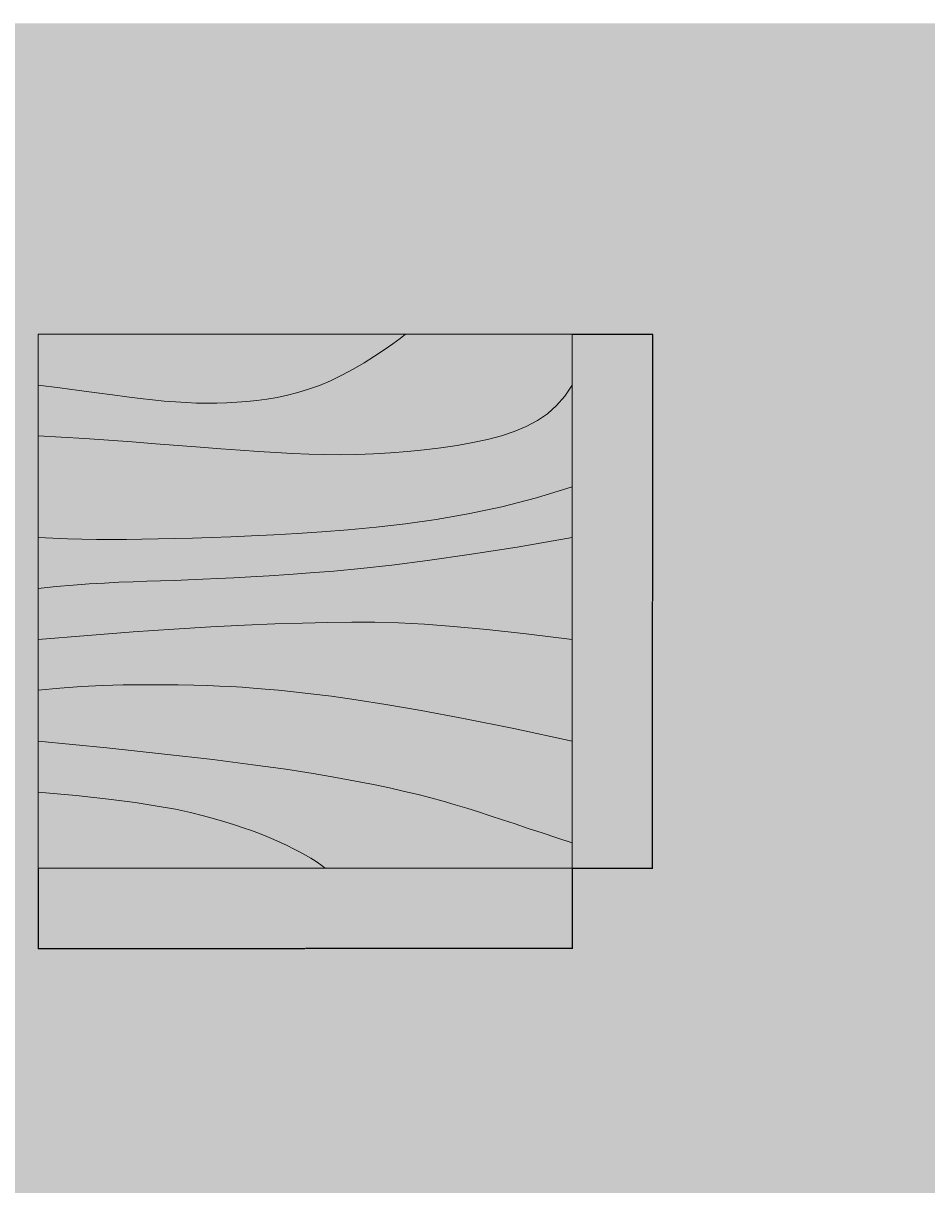
# Model space of a CAD drawing. Units: millimetres. Extents: x -229 to 16545, y -10488 to 4272.
# Tile 24 of 29: x 13075 to 13776, y -2111 to -1208. Entities that reach past the tile are written whole.
import ezdxf

# ---------------------------------------------------------------- set-up
doc = ezdxf.new("R2010")
doc.units = ezdxf.units.MM
for name, color, linetype, lineweight in [('A-ANNO-DIMS', 2, 'Continuous', 18), ('A-FURN', 8, 'Continuous', 18), ('A-FURN-PATT', 252, 'Continuous', 13)]:
    doc.layers.add(name, color=color, linetype=linetype, lineweight=lineweight)
doc.layers.add('A-FLOR-PATT', color=254, linetype='Continuous', lineweight=13, true_color=0xfeeab9)
doc.styles.get("Standard").update_dxf_attribs({"font": 'arial.ttf'})
doc.dimstyles.get("Standard").update_dxf_attribs({"dimtxt": 0.18, "dimasz": 0.18, "dimexe": 0.18, "dimexo": 0.0625, "dimgap": 0.09, "dimtad": 0, "dimtih": 1, "dimtoh": 1, "dimdec": 4, "dimzin": 0, "dimdsep": 46, "dimtxsty": 'Standard', "dimcen": 0.09, "dimadec": 0, "dimazin": 0, "dimtfac": 1, "dimtdec": 4, "dimtofl": 0, "dimtmove": 0, "dimatfit": 3, "dimfxl": 1, "dimtolj": 1, "dimtzin": 0, "dimarcsym": 0})

# ---------------------------------------------------------------- blocks, each defined once
blk = doc.blocks.new('Table - Square Woodgrain 42 x 42 in.')
blk.add_line((0, -42), (42, -42))
for points in [[(0, -4), (1.704, -4.2172), (3.2358, -4.4188), (4.615, -4.604), (5.8615, -4.7721), (6.9951, -4.9224), (8.0357, -5.0541), (9.0031, -5.1667), (9.9171, -5.2594), (10.7951, -5.3316), (11.6445, -5.3836), (12.4702, -5.4157), (13.277, -5.4283), (14.0698, -5.4217), (14.8535, -5.3964), (15.6331, -5.3526), (16.4133, -5.2908), (17.1986, -5.2103), (17.9913, -5.1062), (18.793, -4.9727), (19.6056, -4.8038), (20.4307, -4.5937), (21.2701, -4.3365), (22.1256, -4.0262), (22.9989, -3.6571), (23.888, -3.2272), (24.7756, -2.7516), (25.6408, -2.2491), (26.4624, -1.7387), (27.2195, -1.2395), (27.891, -0.7703), (28.456, -0.3501), (28.8934, 0.002)], [(0, -42), (0, 0), (42, 0), (42, -42)], [(0, -8), (1.8203, -8.1001), (3.6741, -8.2149), (5.5411, -8.3408), (7.4011, -8.4741), (9.2339, -8.6112), (11.0193, -8.7484), (12.7371, -8.8821), (14.3671, -9.0086), (15.8954, -9.1246), (17.3337, -9.2278), (18.6997, -9.3159), (20.0116, -9.387), (21.2871, -9.4389), (22.5442, -9.4696), (23.8008, -9.477), (25.0749, -9.459), (26.3791, -9.4137), (27.7049, -9.3403), (29.0383, -9.2382), (30.3655, -9.1068), (31.6728, -8.9455), (32.9461, -8.7535), (34.1717, -8.5304), (35.3358, -8.2756), (36.4268, -7.9863), (37.443, -7.6521), (38.3849, -7.2603), (39.253, -6.7986), (40.048, -6.2542), (40.7705, -5.6147), (41.421, -4.8674), (42, -4)], [(42, -12), (39.1784, -12.8621), (36.4519, -13.5654), (33.8246, -14.1294), (31.3004, -14.5731), (28.8832, -14.9161), (26.577, -15.1775), (24.3858, -15.3768), (22.3136, -15.5332), (20.3622, -15.6632), (18.5254, -15.7718), (16.7947, -15.8612), (15.1618, -15.9338), (13.6183, -15.9916), (12.1558, -16.0369), (10.7659, -16.0718), (9.4403, -16.0987), (8.1703, -16.1191), (6.9461, -16.1325), (5.7577, -16.1377), (4.595, -16.1335), (3.4479, -16.1188), (2.3064, -16.0924), (1.1604, -16.0532), (0, -16)], [(42, -16), (37.6529, -16.7365), (33.8802, -17.329), (30.6179, -17.7961), (27.8015, -18.1561), (25.3668, -18.4275), (23.2497, -18.6288), (21.3859, -18.7785), (19.7111, -18.8949), (18.1693, -18.9939), (16.7375, -19.0795), (15.401, -19.1534), (14.1449, -19.217), (12.9544, -19.2717), (11.8148, -19.3191), (10.7113, -19.3606), (9.6291, -19.3976), (8.5534, -19.4323), (7.47, -19.4689), (6.3643, -19.5122), (5.222, -19.5672), (4.0288, -19.6386), (2.7703, -19.7313), (1.4321, -19.8501), (0, -20)], [(0, -24), (3.9243, -23.6805), (7.4766, -23.4138), (10.6891, -23.1954), (13.5943, -23.0205), (16.2247, -22.8847), (18.6125, -22.7832), (20.7903, -22.7116), (22.7903, -22.6651), (24.6563, -22.642), (26.4764, -22.6507), (28.35, -22.7024), (30.3766, -22.8084), (32.6555, -22.98), (35.2861, -23.2283), (38.3678, -23.5645), (42, -24)], [(42, -32), (37.392, -31.017), (33.4585, -30.2231), (30.1291, -29.5949), (27.3334, -29.109), (25.0009, -28.742), (23.0612, -28.4707), (21.4439, -28.2716), (20.0786, -28.1215), (18.8998, -28.0002), (17.8609, -27.9014), (16.9206, -27.8219), (16.0371, -27.7588), (15.1691, -27.709), (14.2748, -27.6693), (13.3128, -27.6368), (12.2415, -27.6083), (11.0295, -27.5824), (9.6867, -27.5643), (8.233, -27.5608), (6.6884, -27.5787), (5.0728, -27.6248), (3.4062, -27.7058), (1.7086, -27.8286), (0, -28)], [(0, -32), (5.4026, -32.5358), (9.9494, -33.019), (13.7424, -33.4553), (16.8834, -33.8505), (19.4743, -34.2106), (21.6171, -34.5413), (23.4136, -34.8486), (24.9657, -35.1382), (26.3614, -35.4156), (27.6332, -35.6841), (28.7995, -35.9467), (29.8788, -36.2064), (30.8897, -36.4661), (31.8507, -36.7288), (32.7802, -36.9973), (33.6968, -37.2747), (34.6175, -37.5635), (35.5531, -37.8651), (36.5128, -38.1805), (37.506, -38.5108), (38.5421, -38.8568), (39.6302, -39.2197), (40.7797, -39.6004), (42, -40)], [(0, -36), (3.0098, -36.2857), (5.5354, -36.5643), (7.6368, -36.8359), (9.374, -37.1009), (10.807, -37.3597), (11.9957, -37.6126), (13.0002, -37.8599), (13.8804, -38.102), (14.6874, -38.3393), (15.4365, -38.5729), (16.1338, -38.8041), (16.7858, -39.0341), (17.3987, -39.264), (17.9787, -39.4952), (18.5322, -39.7288), (19.0655, -39.9662), (19.5832, -40.2081), (20.0842, -40.4544), (20.5657, -40.7046), (21.0249, -40.9581), (21.459, -41.2144), (21.8653, -41.4731), (22.2409, -41.7335), (22.5831, -41.9951)]]:
    blk.add_lwpolyline(points)
blk = doc.blocks.new('*D43')
at = {"layer": 'A-ANNO-DIMS', "color": 0, "lineweight": -2, "transparency": 16777216}
for p, q in [((13501.11, -1449.82), (13563.48, -1449.82)), ((13563.3, -1450), (13563.3, -1657.14)), ((13563.3, -1864.65), (13563.3, -1657.51)), ((13501.11, -1864.83), (13563.48, -1864.83))]:
    blk.add_line(p, q, dxfattribs=at)
at = {"layer": 'A-ANNO-DIMS', "color": 0, "transparency": 16777216}
for points in [[(13563.27, -1450), (13563.33, -1450), (13563.3, -1449.82)], [(13563.27, -1864.65), (13563.33, -1864.65), (13563.3, -1864.83)]]:
    blk.add_solid(points, dxfattribs=at)
at = {"layer": 'Defpoints', "color": 0, "transparency": 16777216}
for p in [(13501.05, -1449.82), (13563.3, -1449.82), (13501.05, -1864.83)]:
    blk.add_point(p, dxfattribs=at)
at = {"layer": 'A-ANNO-DIMS', "color": 0, "transparency": 16777216, "insert": (13563.3, -1657.33), "char_height": 0.18, "attachment_point": 5}
blk.add_mtext('\\A1;END TABLE 415', dxfattribs=at)
blk = doc.blocks.new('*D44')
at = {"layer": 'A-ANNO-DIMS', "color": 0, "lineweight": -2, "transparency": 16777216}
for p, q in [((13086.06, -1864.89), (13086.06, -1927.26)), ((13501.05, -1864.89), (13501.05, -1927.26)), ((13086.24, -1927.08), (13293.26, -1927.08)), ((13500.87, -1927.08), (13293.85, -1927.08))]:
    blk.add_line(p, q, dxfattribs=at)
at = {"layer": 'A-ANNO-DIMS', "color": 0, "transparency": 16777216}
for points in [[(13086.24, -1927.05), (13086.24, -1927.11), (13086.06, -1927.08)], [(13500.87, -1927.05), (13500.87, -1927.11), (13501.05, -1927.08)]]:
    blk.add_solid(points, dxfattribs=at)
at = {"layer": 'Defpoints', "color": 0, "transparency": 16777216}
for p in [(13086.06, -1864.83), (13501.05, -1864.83), (13501.05, -1927.08)]:
    blk.add_point(p, dxfattribs=at)
at = {"layer": 'A-ANNO-DIMS', "color": 0, "transparency": 16777216, "insert": (13293.55, -1927.08), "char_height": 0.18, "attachment_point": 5}
blk.add_mtext('\\A1;415', dxfattribs=at)

msp = doc.modelspace()

# ---------------------------------------------------------------- hatches: boundary and pattern name
at = {"layer": 'A-FLOR-PATT', "transparency": 33554592}
h = msp.add_hatch(color=256, dxfattribs=at)
h.dxf.hatch_style = 1
h.paths.add_polyline_path([(7975.933, -5325.772), (7943.121, -5325.772), (7943.121, -4576.49, 0.4014527), (7225.933, -5325.772, 0.4014527), (6508.746, -4576.49), (6508.746, -5325.772), (6475.933, -5325.772), (6475.933, -5438.272), (5975.933, -5438.272), (5975.933, -7267.724), (5975.933, -7438.272), (6478.619, -7438.272), (6463.448, -7355.919), (6464.88, -7356.837), (6463.849, -7358.097), (6478.619, -7438.272), (6610.327, -7438.272), (6632.656, -7409.564), (6632.525, -7406.967), (6634.208, -7407.569), (6619.273, -7426.77), (6654.466, -7438.272), (7610.517, -7438.272), (7607.41, -7421.409), (7608.842, -7422.327), (7607.812, -7423.587), (7610.517, -7438.272), (7975.933, -7438.272)])
h.paths.add_polyline_path([(13785.933, -1208.272), (9555.933, -1208.272), (9555.933, -961.785), (9705.933, -961.785), (9705.933, -918.035), (10704.976, -918.035, 0.4014527), (9705.933, 38.215), (9555.933, 38.215), (9555.933, 2021.728), (5975.933, 2021.728), (5975.933, 755.492), (5745.933, 755.492), (5745.933, 1427.266), (2918.813, 1427.266), (2918.813, -492.942), (5013.319, -492.942), (5013.319, -978.272), (5745.933, -978.272), (5745.933, -397.513), (5975.933, -397.513), (5975.933, -1208.272), (4560.933, -1208.272), (4560.933, -1265.772), (4448.433, -1265.772), (4448.433, -1298.585), (4445.933, -1298.585), (3699.151, -1298.585, 0.4014527), (4448.433, -2015.772), (4560.933, -2015.772), (4560.933, -2384.177), (5745.933, -2384.177), (5799.402, -2384.177), (5799.402, -4518.272), (5975.933, -4518.272), (5975.933, -5208.272), (6475.933, -5208.272), (6475.933, -4575.772), (6508.746, -4575.772), (6508.746, -4576.49, -0.3564726), (7216.672, -5208.272), (7235.194, -5208.272, -0.3564726), (7943.121, -4576.49), (7943.121, -4575.772), (7975.933, -4575.772), (7975.933, -5208.272), (11176.247, -5208.272), (11159.44, -5191.465), (10520.768, -5191.465), (10520.768, -4888.936), (10571.19, -4888.936), (10571.19, -4872.129), (10772.876, -4872.129), (10772.876, -4888.936), (10789.683, -4888.936), (10789.683, -4872.129), (10991.368, -4872.129), (10991.368, -4888.936), (11041.79, -4888.936), (11041.79, -4872.129), (11058.597, -4872.129, -0.0909091), (11428.354, -4872.129), (11445.162, -4872.129), (11445.162, -4888.936), (11529.197, -4888.936), (11529.197, -5191.465), (11327.512, -5191.465), (11310.704, -5208.272), (13785.933, -5208.272)])
h.paths.add_polyline_path([(11047.216, -1630.944, -1), (11402.816, -1630.944, -1)], flags=16)
h.paths.add_polyline_path([(11148.816, -1630.944), (11225.016, -1554.744), (11301.216, -1630.944), (11225.016, -1707.144)], flags=0)
h.paths.add_polyline_path([(11199.616, -1630.944, -1), (11250.416, -1630.944, -1)], flags=0)
h.paths.add_polyline_path([(11588.751, -2096.259), (11588.751, -1543.254, -0.266667), (12864.918, -1543.254), (12864.918, -2096.259), (12737.302, -2096.259), (12737.302, -2063.121), (11716.368, -2063.121), (11716.368, -2096.259)], flags=16)
h.paths.add_polyline_path([(12012.696, -2489.42), (12600.997, -2489.42), (12600.997, -3666.022), (12012.696, -3666.022)], flags=16)
h.paths.add_polyline_path([(12176.41, -3599.403), (12174.938, -3609.076), (12173.789, -3618.819), (12173.09, -3628.559), (12172.973, -3638.221), (12173.89, -3652.852), (12175.008, -3657.025), (12172.909, -3643.473), (12173.142, -3624.297), (12175.386, -3605.273)], flags=0)
h.paths.add_polyline_path([(8026.289, -286.944), (7737.703, -287.19), (7734.87, -269.156), (8029.092, -268.905)], flags=16)
h.paths.add_polyline_path([(7733.453, -260.139), (7710.784, -115.865), (7557.191, -115.996), (7556.999, 109.744), (7412.687, 132.166), (7412.433, 429.206), (7556.707, 451.876), (7556.568, 614.769), (7412.256, 637.19), (7412.003, 934.231), (7556.276, 956.9), (7556.084, 1182.639), (7709.677, 1182.77), (7732.099, 1327.082), (8029.14, 1327.335), (8051.808, 1183.062), (8205.401, 1183.192), (8205.594, 957.454), (8349.906, 935.031), (8350.159, 637.99), (8205.885, 615.322), (8206.024, 452.43), (8350.336, 430.006), (8350.59, 132.965), (8206.316, 110.298), (8206.509, -115.442), (8052.916, -115.573), (8030.493, -259.885)], flags=16)
h.paths.add_polyline_path([(12261.416, -3475.554), (12262.632, -3486.776), (12264.032, -3497.007), (12265.554, -3506.365), (12267.136, -3514.968), (12268.719, -3522.935), (12271.304, -3535.59), (12273.606, -3548.078), (12275.271, -3561.064), (12275.93, -3574.938), (12275.325, -3590.3), (12273.425, -3607.964), (12270.795, -3625.658), (12268.066, -3641.063), (12266.318, -3649.679), (12265.456, -3653.626), (12263.984, -3659.846), (12264.032, -3659.566), (12264.342, -3658.241), (12264.807, -3656.37), (12265.456, -3653.626), (12266.318, -3649.679), (12267.409, -3644.302), (12268.668, -3637.664), (12270.019, -3630.037), (12271.384, -3621.695), (12272.69, -3612.908), (12273.857, -3603.948), (12274.81, -3595.088), (12275.47, -3586.601), (12275.782, -3578.689), (12275.757, -3571.292), (12275.423, -3564.275), (12274.816, -3557.512), (12273.964, -3550.872), (12272.896, -3544.224), (12271.645, -3537.439), (12270.24, -3530.385), (12267.543, -3517.181), (12264.612, -3501.247), (12261.849, -3481.059)], flags=0)
h.paths.add_polyline_path([(12332.136, -3408.03), (12333.483, -3416.79), (12335.077, -3424.54), (12336.915, -3431.355), (12338.991, -3437.32), (12341.266, -3442.55), (12343.694, -3447.166), (12346.229, -3451.292), (12348.826, -3455.051), (12351.438, -3458.563), (12357.476, -3466.491), (12363.61, -3476.575), (12368.309, -3489.762), (12369.929, -3503.427), (12369.842, -3516.511), (12368.43, -3530.867), (12365.816, -3545.835), (12362.382, -3559.786), (12360.968, -3564.487), (12363.063, -3557.021), (12364.898, -3549.566), (12366.473, -3542.077), (12367.773, -3534.631), (12368.781, -3527.301), (12369.483, -3520.162), (12369.863, -3513.291), (12369.906, -3506.759), (12369.599, -3500.643), (12368.93, -3494.999), (12367.924, -3489.796), (12366.61, -3484.994), (12365.024, -3480.542), (12363.19, -3476.399), (12361.141, -3472.516), (12358.909, -3468.847), (12356.525, -3465.347), (12354.02, -3461.954), (12351.438, -3458.563), (12345.462, -3450.529), (12339.923, -3439.996), (12335.85, -3428.296), (12332.68, -3412.888)], flags=0)
h.paths.add_polyline_path([(12385.287, -3334.612), (12384.977, -3342.409), (12385.02, -3349.196), (12385.4, -3355.066), (12386.104, -3360.105), (12387.112, -3364.41), (12388.412, -3368.071), (12389.987, -3371.181), (12391.823, -3373.832), (12393.919, -3376.097), (12396.337, -3377.978), (12399.153, -3379.462), (12402.445, -3380.531), (12406.289, -3381.172), (12410.758, -3381.371), (12415.935, -3381.106), (12421.893, -3380.368), (12428.658, -3379.159), (12436.069, -3377.55), (12443.907, -3375.635), (12451.961, -3373.505), (12460.015, -3371.254), (12467.853, -3368.971), (12475.263, -3366.749), (12482.029, -3364.68), (12491.877, -3361.657), (12497.701, -3360.107), (12501.639, -3359.288), (12510.135, -3358.326), (12519.662, -3365.412), (12524.243, -3378.911), (12523.764, -3390.7), (12520.746, -3401.577), (12514.248, -3415.634), (12511.518, -3420.418), (12515.856, -3412.154), (12519.153, -3405.024), (12521.516, -3398.804), (12523.049, -3393.276), (12523.865, -3388.212), (12524.059, -3383.441), (12523.7, -3378.958), (12522.853, -3374.815), (12521.576, -3371.054), (12519.931, -3367.722), (12517.982, -3364.865), (12515.786, -3362.529), (12513.405, -3360.758), (12510.877, -3359.588), (12508.136, -3358.982), (12505.086, -3358.897), (12501.639, -3359.288), (12497.701, -3360.107), (12493.183, -3361.309), (12487.988, -3362.851), (12476.403, -3366.408), (12463.335, -3370.326), (12447.372, -3374.788), (12431.759, -3378.604), (12418.504, -3380.974), (12405.811, -3381.624), (12394.725, -3378.025), (12388.039, -3368.367), (12385.583, -3357.877), (12384.826, -3346.204), (12385.428, -3331.059), (12385.953, -3325.719)], flags=0)
h.paths.add_polyline_path([(7880.016, 1173.969), (7880.373, 1175.495), (7880.433, 1175.851), (7879.484, 1171.818)], flags=0)
h.paths.add_polyline_path([(7802.33, 874.962), (7800.771, 885.032), (7798.932, 893.941), (7796.811, 901.774), (7794.419, 908.63), (7791.798, 914.639), (7789.002, 919.945), (7786.083, 924.686), (7783.093, 929.005), (7780.087, 933.043), (7774.996, 939.717), (7768.406, 949.37), (7762.174, 963.427), (7759.342, 978.002), (7758.629, 991.888), (7759.492, 1007.928), (7761.801, 1025.496), (7765.392, 1044.035), (7766.625, 1049.048), (7764.522, 1039.543), (7762.719, 1030.232), (7761.232, 1021.168), (7760.08, 1012.405), (7759.28, 1003.994), (7758.849, 995.988), (7758.806, 988.44), (7759.167, 981.404), (7759.942, 974.914), (7761.104, 968.936), (7762.617, 963.414), (7764.448, 958.299), (7766.559, 953.535), (7768.918, 949.073), (7771.487, 944.856), (7774.232, 940.835), (7777.115, 936.938), (7782.377, 930.041), (7787.845, 922.139), (7793.348, 911.698), (7798.042, 898.247), (7801.702, 880.527)], flags=0)
h.paths.add_polyline_path([(12519.068, -3228.534), (12519.615, -3236.235), (12520.529, -3242.343), (12521.78, -3247.103), (12523.337, -3250.758), (12525.171, -3253.556), (12527.248, -3255.709), (12529.522, -3257.296), (12531.95, -3258.361), (12534.486, -3258.949), (12537.082, -3259.11), (12539.694, -3258.888), (12542.277, -3258.329), (12544.781, -3257.478), (12547.173, -3256.388), (12549.46, -3255.129), (12550.455, -3254.517), (12555.825, -3251.109), (12557.835, -3249.942), (12565.181, -3246.404), (12574.565, -3253.032), (12576.931, -3265.022), (12576.627, -3277.425), (12575.416, -3290.819), (12574.851, -3295.392), (12575.708, -3287.593), (12576.322, -3280.806), (12576.688, -3274.939), (12576.812, -3269.899), (12576.688, -3265.593), (12576.322, -3261.932), (12575.708, -3258.822), (12574.851, -3256.172), (12573.753, -3253.905), (12572.439, -3252.005), (12570.943, -3250.474), (12569.293, -3249.309), (12567.523, -3248.513), (12565.658, -3248.083), (12563.732, -3248.022), (12561.777, -3248.328), (12559.814, -3248.989), (12557.835, -3249.942), (12555.825, -3251.109), (12553.77, -3252.413), (12551.652, -3253.78), (12549.46, -3255.129), (12543.167, -3258.594), (12532.661, -3259.485), (12524.685, -3253.923), (12520.949, -3245.152), (12519.138, -3233.042)], flags=0)
h.paths.add_polyline_path([(7741.293, 790.501), (7741.641, 799.467), (7741.584, 807.269), (7741.141, 814.015), (7740.329, 819.809), (7739.165, 824.757), (7737.667, 828.966), (7735.853, 832.541), (7733.74, 835.586), (7731.348, 838.188), (7728.71, 840.348), (7725.861, 842.052), (7722.836, 843.28), (7719.671, 844.015), (7716.4, 844.237), (7713.06, 843.932), (7709.684, 843.081), (7706.304, 841.686), (7702.923, 839.834), (7699.543, 837.629), (7696.164, 835.178), (7692.784, 832.585), (7684.718, 826.315), (7675.609, 820.63), (7664.001, 817.274), (7654.105, 821.884), (7647.171, 832.02), (7644.191, 846.522), (7646.321, 860.288), (7647.49, 864.223), (7645.946, 857.865), (7645.046, 852.044), (7644.827, 846.557), (7645.243, 841.404), (7646.221, 836.642), (7647.693, 832.318), (7649.587, 828.489), (7651.832, 825.206), (7654.359, 822.523), (7657.097, 820.49), (7659.984, 819.145), (7662.993, 818.452), (7666.108, 818.357), (7669.311, 818.809), (7672.583, 819.755), (7675.908, 821.139), (7679.268, 822.913), (7682.645, 825.021), (7686.025, 827.401), (7689.404, 829.958), (7692.784, 832.585), (7700.505, 838.509), (7709.871, 843.64), (7721.436, 844.698), (7733.277, 837.617), (7739.571, 825.214), (7741.557, 811.049), (7741.669, 795.575)], flags=0)
h.paths.add_polyline_path([(8377.641, 137.216), (8359.607, 134.382), (8359.356, 428.605), (8377.395, 425.802)], flags=16)
h.paths.add_polyline_path([(7650.715, 668.465), (7650.08, 677.319), (7649.023, 684.34), (7647.579, 689.811), (7645.785, 694.012), (7643.675, 697.228), (7641.286, 699.7), (7638.669, 701.521), (7635.876, 702.744), (7632.96, 703.419), (7629.974, 703.601), (7626.971, 703.344), (7624.004, 702.697), (7621.125, 701.717), (7618.375, 700.462), (7615.749, 699.013), (7614.561, 698.279), (7608.435, 694.382), (7606.125, 693.04), (7598.981, 689.594), (7589.669, 693.773), (7585.26, 702.856), (7584.221, 713.11), (7584.49, 724.584), (7585.863, 739.937), (7586.518, 745.277), (7585.539, 736.31), (7584.841, 728.507), (7584.424, 721.761), (7584.288, 715.966), (7584.433, 711.016), (7584.86, 706.807), (7585.567, 703.231), (7586.556, 700.186), (7587.821, 697.58), (7589.332, 695.397), (7591.053, 693.637), (7592.951, 692.3), (7594.989, 691.385), (7597.132, 690.895), (7599.346, 690.826), (7601.594, 691.18), (7603.851, 691.943), (7606.125, 693.04), (7608.435, 694.382), (7610.797, 695.885), (7613.229, 697.458), (7620.475, 701.929), (7632.001, 704.44), (7643.476, 699.417), (7648.536, 687.571), (7650.63, 673.661)], flags=0)
h.paths.add_polyline_path([(7385.628, 136.37), (7385.382, 424.956), (7403.416, 427.789), (7403.667, 133.567)], flags=16)
h.paths.add_polyline_path([(12993.884, -2257.186), (12959.588, -2257.186), (12959.588, -2125.099), (13531.966, -2125.099, -0.1904762), (13531.966, -3974.321), (12959.588, -3974.321), (12959.588, -3842.233), (12993.884, -3842.233)], flags=16)
h.paths.add_polyline_path([(13413.486, -3313.884), (13413.486, -2785.535), (13562.885, -2785.535, -0.0496282), (13562.885, -3313.884)], flags=0)
h.paths.add_polyline_path([(8377.21, 642.241), (8359.176, 639.407), (8358.925, 933.629), (8376.964, 930.826)], flags=16)
h.paths.add_polyline_path([(13086.058, -1864.83), (13086.058, -1449.84), (13501.048, -1449.84), (13501.048, -1864.83)], flags=16)
h.paths.add_polyline_path([(13305.814, -1862.197), (13302.103, -1859.624), (13298.088, -1857.068), (13293.799, -1854.536), (13289.262, -1852.031), (13284.504, -1849.559), (13279.554, -1847.125), (13274.439, -1844.735), (13269.17, -1842.389), (13263.701, -1840.081), (13257.97, -1837.797), (13251.914, -1835.525), (13245.472, -1833.252), (13238.582, -1830.968), (13231.18, -1828.66), (13223.206, -1826.315), (13209.182, -1822.458), (13204.584, -1821.48), (13217.962, -1824.773), (13235.072, -1829.804), (13248.777, -1834.349), (13260.829, -1838.869), (13274.479, -1844.63), (13289.675, -1852.101), (13302.553, -1859.704)], flags=0)
h.paths.add_polyline_path([(13428.104, -1820.994), (13419.007, -1818.141), (13409.95, -1815.4), (13400.766, -1812.747), (13391.271, -1810.151), (13376.087, -1806.251), (13370.618, -1805.019), (13386.304, -1808.794), (13405.087, -1813.928), (13423.014, -1819.354)], flags=0)
h.paths.add_polyline_path([(7385.197, 641.395), (7384.951, 929.98), (7402.986, 932.814), (7403.236, 638.592)], flags=16)
h.paths.add_polyline_path([(13262.537, -1725.526), (13253.246, -1724.74), (13244.516, -1724.117), (13235.94, -1723.625), (13223.267, -1723.062), (13217.598, -1722.912), (13231.966, -1723.397), (13248.733, -1724.359), (13266.899, -1725.895), (13272.802, -1726.502)], flags=0)
h.paths.add_polyline_path([(13191.893, -1641.137), (13208.675, -1640.506), (13214.057, -1640.258), (13197.763, -1640.936)], flags=0)
h.paths.add_polyline_path([(13097.524, -1608.457), (13114.284, -1609.031), (13120.126, -1609.105), (13103.045, -1608.71)], flags=0)
h.paths.add_polyline_path([(13465.328, -1521.577), (13473.906, -1517.015), (13481.761, -1511.636), (13492.562, -1502.076), (13495.327, -1497.933), (13485.818, -1508.858), (13470.208, -1519.547)], flags=0)
h.paths.add_polyline_path([(13175.015, -1500.891), (13184.046, -1501.807), (13192.721, -1502.52), (13201.114, -1503.034), (13209.273, -1503.351), (13217.244, -1503.476), (13225.078, -1503.41), (13232.821, -1503.16), (13240.524, -1502.728), (13248.233, -1502.117), (13255.993, -1501.322), (13263.825, -1500.293), (13271.746, -1498.974), (13279.775, -1497.305), (13287.928, -1495.229), (13296.222, -1492.688), (13304.675, -1489.622), (13313.304, -1485.975), (13322.089, -1481.727), (13330.859, -1477.028), (13339.408, -1472.063), (13347.526, -1467.02), (13355.006, -1462.087), (13364.86, -1455.202), (13367.224, -1453.299), (13358.544, -1459.754), (13343.348, -1469.775), (13326.143, -1479.767), (13309.023, -1488.045), (13292.249, -1494.129), (13276.009, -1498.264), (13260.299, -1500.88), (13244.401, -1502.51), (13228.945, -1503.378), (13213.316, -1503.508), (13197.047, -1502.876), (13180.088, -1501.481)], flags=0)
h.paths.add_polyline_path([(7733.501, 1336.101), (7736.303, 1354.14), (8024.889, 1354.386), (8027.723, 1336.352)], flags=16)
at = {"layer": 'A-FURN-PATT', "transparency": 33554569}
h = msp.add_hatch(color=256, dxfattribs=at)
h.dxf.hatch_style = 1
h.paths.add_polyline_path([(12600.997, -2489.42), (12553.933, -2489.42), (12553.58, -2583.852), (12552.584, -2666.503), (12551.036, -2738.644), (12549.03, -2801.547), (12546.656, -2856.483), (12544.004, -2904.723), (12541.171, -2947.542), (12538.245, -2986.207), (12535.313, -3021.787), (12532.444, -3054.526), (12529.695, -3084.461), (12527.132, -3111.629), (12524.814, -3136.073), (12522.802, -3157.826), (12521.157, -3176.928), (12519.941, -3193.42), (12519.202, -3207.371), (12518.921, -3218.994), (12519.068, -3228.534), (12519.615, -3236.235), (12520.529, -3242.343), (12521.78, -3247.103), (12523.337, -3250.758), (12525.171, -3253.556), (12527.248, -3255.709), (12529.522, -3257.296), (12531.95, -3258.361), (12534.486, -3258.949), (12537.082, -3259.11), (12539.694, -3258.888), (12542.277, -3258.329), (12544.781, -3257.478), (12547.173, -3256.388), (12549.46, -3255.129), (12551.652, -3253.78), (12559.563, -3248.675), (12566.794, -3247.543), (12572.687, -3251.706), (12575.978, -3258.498), (12576.872, -3267.431), (12576.627, -3277.425), (12575.708, -3287.593), (12574.851, -3295.392), (12573.749, -3304.309), (12572.419, -3314.522), (12570.874, -3326.221), (12569.131, -3339.597), (12567.203, -3354.842), (12565.107, -3372.146), (12562.857, -3391.705), (12560.469, -3413.705), (12557.959, -3438.275), (12555.343, -3465.264), (12552.633, -3494.46), (12549.848, -3525.645), (12547.001, -3558.61), (12544.106, -3593.137), (12541.184, -3629.012), (12538.245, -3666.022), (12600.997, -3666.022)])
h.paths.add_polyline_path([(12544.004, -2904.723), (12546.656, -2856.483), (12549.03, -2801.547), (12551.036, -2738.644), (12552.584, -2666.503), (12553.58, -2583.852), (12553.933, -2489.42), (12420.585, -2489.42), (12422.824, -2618.374), (12423.791, -2723.534), (12423.687, -2808.136), (12422.708, -2875.41), (12421.057, -2928.591), (12418.93, -2970.907), (12416.527, -3005.595), (12414.049, -3035.885), (12411.656, -3064.467), (12409.37, -3091.846), (12407.177, -3117.984), (12405.059, -3142.842), (12403.004, -3166.384), (12400.994, -3188.569), (12399.016, -3209.359), (12397.053, -3228.718), (12395.1, -3246.62), (12393.191, -3263.097), (12391.376, -3278.194), (12389.699, -3291.961), (12388.205, -3304.438), (12386.942, -3315.677), (12385.953, -3325.719), (12385.287, -3334.612), (12384.977, -3342.409), (12385.02, -3349.196), (12385.4, -3355.066), (12386.104, -3360.105), (12387.112, -3364.41), (12388.412, -3368.071), (12389.987, -3371.181), (12391.823, -3373.832), (12393.919, -3376.097), (12396.337, -3377.978), (12399.153, -3379.462), (12402.445, -3380.531), (12406.289, -3381.172), (12410.758, -3381.371), (12415.935, -3381.106), (12421.893, -3380.368), (12428.658, -3379.159), (12436.069, -3377.55), (12443.907, -3375.635), (12451.961, -3373.505), (12460.015, -3371.254), (12467.853, -3368.971), (12475.263, -3366.749), (12482.029, -3364.68), (12491.877, -3361.657), (12502.516, -3358.826), (12511.128, -3359.064), (12517.01, -3363.44), (12520.955, -3369.223), (12523.527, -3376.802), (12524.25, -3385.824), (12522.632, -3395.865), (12519.153, -3405.024), (12515.856, -3412.154), (12511.518, -3420.418), (12506.031, -3430.037), (12499.288, -3441.236), (12491.181, -3454.234), (12481.682, -3469.286), (12471.081, -3486.774), (12459.744, -3507.112), (12448.039, -3530.713), (12436.334, -3557.99), (12424.997, -3589.358), (12414.396, -3625.231), (12404.897, -3666.022), (12538.245, -3666.022), (12541.184, -3629.012), (12544.106, -3593.137), (12547.001, -3558.61), (12549.848, -3525.645), (12552.633, -3494.46), (12555.343, -3465.264), (12557.959, -3438.275), (12560.469, -3413.705), (12562.857, -3391.705), (12565.107, -3372.146), (12567.203, -3354.842), (12569.131, -3339.597), (12570.874, -3326.221), (12572.419, -3314.522), (12573.749, -3304.309), (12574.851, -3295.392), (12575.708, -3287.593), (12576.322, -3280.806), (12576.688, -3274.939), (12576.812, -3269.899), (12576.688, -3265.593), (12576.322, -3261.932), (12575.708, -3258.822), (12574.851, -3256.172), (12573.753, -3253.905), (12572.439, -3252.005), (12570.943, -3250.474), (12569.293, -3249.309), (12567.523, -3248.513), (12565.658, -3248.083), (12563.732, -3248.022), (12561.777, -3248.328), (12559.814, -3248.989), (12557.835, -3249.942), (12555.825, -3251.109), (12553.77, -3252.413), (12547.19, -3256.659), (12539.533, -3259.262), (12531.64, -3258.773), (12524.685, -3253.923), (12520.949, -3245.152), (12519.615, -3236.235), (12519.068, -3228.534), (12518.921, -3218.994), (12519.202, -3207.371), (12519.941, -3193.42), (12521.157, -3176.928), (12522.802, -3157.826), (12524.814, -3136.073), (12527.132, -3111.629), (12529.695, -3084.461), (12532.444, -3054.526), (12535.313, -3021.787), (12538.245, -2986.207), (12541.171, -2947.542)])
h.paths.add_polyline_path([(12418.93, -2970.907), (12421.057, -2928.591), (12422.708, -2875.41), (12423.687, -2808.136), (12423.791, -2723.534), (12422.824, -2618.374), (12420.585, -2489.42), (12349.989, -2489.42), (12347.396, -2591.092), (12345.433, -2678.094), (12343.99, -2752.122), (12342.962, -2814.864), (12342.239, -2868.017), (12341.715, -2913.271), (12341.284, -2952.323), (12340.837, -2986.86), (12340.288, -3018.358), (12339.633, -3047.386), (12338.883, -3074.301), (12338.06, -3099.455), (12337.173, -3123.199), (12336.242, -3145.885), (12335.279, -3167.868), (12334.301, -3189.498), (12333.326, -3211.038), (12332.381, -3232.395), (12331.496, -3253.384), (12330.706, -3273.821), (12330.037, -3293.523), (12329.52, -3312.306), (12329.188, -3329.984), (12329.071, -3346.378), (12329.194, -3361.343), (12329.561, -3374.915), (12330.175, -3387.169), (12331.032, -3398.18), (12332.136, -3408.03), (12333.483, -3416.79), (12335.077, -3424.54), (12336.915, -3431.355), (12338.991, -3437.32), (12341.266, -3442.55), (12343.694, -3447.166), (12346.229, -3451.292), (12348.826, -3455.051), (12351.438, -3458.563), (12357.476, -3466.491), (12362.356, -3474.514), (12365.989, -3482.725), (12368.611, -3492.308), (12369.929, -3503.427), (12369.863, -3513.291), (12369.483, -3520.162), (12368.781, -3527.301), (12367.773, -3534.631), (12366.473, -3542.077), (12364.898, -3549.566), (12363.063, -3557.021), (12360.968, -3564.487), (12358.568, -3572.468), (12355.799, -3581.585), (12352.603, -3592.463), (12348.916, -3605.723), (12344.678, -3621.988), (12339.827, -3641.88), (12334.301, -3666.022), (12404.897, -3666.022), (12414.396, -3625.231), (12424.997, -3589.358), (12436.334, -3557.99), (12448.039, -3530.713), (12459.744, -3507.112), (12471.081, -3486.774), (12481.682, -3469.286), (12491.181, -3454.234), (12499.288, -3441.236), (12506.031, -3430.037), (12511.518, -3420.418), (12515.856, -3412.154), (12519.153, -3405.024), (12521.516, -3398.804), (12523.049, -3393.276), (12523.865, -3388.212), (12524.059, -3383.441), (12523.7, -3378.958), (12522.853, -3374.815), (12521.576, -3371.054), (12519.931, -3367.722), (12517.982, -3364.865), (12515.786, -3362.529), (12513.405, -3360.758), (12510.877, -3359.588), (12508.136, -3358.982), (12505.086, -3358.897), (12501.639, -3359.288), (12497.701, -3360.107), (12493.183, -3361.309), (12487.988, -3362.851), (12476.403, -3366.408), (12463.335, -3370.326), (12451.961, -3373.505), (12439.372, -3376.834), (12424.661, -3380.026), (12412.995, -3381.47), (12402.039, -3380.984), (12393.748, -3376.613), (12389.022, -3369.787), (12386.442, -3362.522), (12385.041, -3352.492), (12384.977, -3342.409), (12385.287, -3334.612), (12385.953, -3325.719), (12386.942, -3315.677), (12388.205, -3304.438), (12389.699, -3291.961), (12391.376, -3278.194), (12393.191, -3263.097), (12395.1, -3246.62), (12397.053, -3228.718), (12399.016, -3209.359), (12400.994, -3188.569), (12403.004, -3166.384), (12405.059, -3142.842), (12407.177, -3117.984), (12409.37, -3091.846), (12411.656, -3064.467), (12414.049, -3035.885), (12416.527, -3005.595)])
h.paths.add_polyline_path([(12340.837, -2986.86), (12341.284, -2952.323), (12341.715, -2913.271), (12342.239, -2868.017), (12342.962, -2814.864), (12343.99, -2752.122), (12345.433, -2678.094), (12347.396, -2591.092), (12349.989, -2489.42), (12248.016, -2489.42), (12253.364, -2589.902), (12257.71, -2678.871), (12261.149, -2757.499), (12263.787, -2826.958), (12265.718, -2888.42), (12267.044, -2943.055), (12267.866, -2992.039), (12268.279, -3036.54), (12268.378, -3077.58), (12268.209, -3115.572), (12267.809, -3150.776), (12267.219, -3183.452), (12266.473, -3213.86), (12265.614, -3242.261), (12264.679, -3268.917), (12263.704, -3294.084), (12262.732, -3317.981), (12261.804, -3340.639), (12260.969, -3362.039), (12260.273, -3382.167), (12259.759, -3401.008), (12259.477, -3418.547), (12259.469, -3434.769), (12259.782, -3449.659), (12260.445, -3463.221), (12261.416, -3475.554), (12262.632, -3486.776), (12264.032, -3497.007), (12265.554, -3506.365), (12267.136, -3514.968), (12268.719, -3522.935), (12271.304, -3535.59), (12273.606, -3548.078), (12275.271, -3561.064), (12275.757, -3571.292), (12275.782, -3578.689), (12275.47, -3586.601), (12274.81, -3595.088), (12273.857, -3603.948), (12272.69, -3612.908), (12271.384, -3621.695), (12270.019, -3630.037), (12268.066, -3641.063), (12265.651, -3652.97), (12264.342, -3658.241), (12264.032, -3659.566), (12263.842, -3660.678), (12263.746, -3661.906), (12263.708, -3663.576), (12263.704, -3666.022), (12334.301, -3666.022), (12339.827, -3641.88), (12344.678, -3621.988), (12348.916, -3605.723), (12352.603, -3592.463), (12355.799, -3581.585), (12358.568, -3572.468), (12360.968, -3564.487), (12363.063, -3557.021), (12364.898, -3549.566), (12366.473, -3542.077), (12367.773, -3534.631), (12368.781, -3527.301), (12369.483, -3520.162), (12369.863, -3513.291), (12369.906, -3506.759), (12369.599, -3500.643), (12368.93, -3494.999), (12367.924, -3489.796), (12366.61, -3484.994), (12365.024, -3480.542), (12363.19, -3476.399), (12361.141, -3472.516), (12358.909, -3468.847), (12356.525, -3465.347), (12354.02, -3461.954), (12347.609, -3453.536), (12342.257, -3444.828), (12337.759, -3434.488), (12335.077, -3424.54), (12333.483, -3416.79), (12332.136, -3408.03), (12331.032, -3398.18), (12330.175, -3387.169), (12329.561, -3374.915), (12329.194, -3361.343), (12329.071, -3346.378), (12329.188, -3329.984), (12329.52, -3312.306), (12330.037, -3293.523), (12330.706, -3273.821), (12331.496, -3253.384), (12332.381, -3232.395), (12333.326, -3211.038), (12334.301, -3189.498), (12335.279, -3167.868), (12336.242, -3145.885), (12337.173, -3123.199), (12338.06, -3099.455), (12338.883, -3074.301), (12339.633, -3047.386), (12340.288, -3018.358)])
h.paths.add_polyline_path([(12267.866, -2992.039), (12267.044, -2943.055), (12265.718, -2888.42), (12263.787, -2826.958), (12261.149, -2757.499), (12257.71, -2678.871), (12253.364, -2589.902), (12248.016, -2489.42), (12161.732, -2489.42), (12164.672, -2646.493), (12167.594, -2771.989), (12170.488, -2870.184), (12173.336, -2945.353), (12176.12, -3001.769), (12178.83, -3043.709), (12181.446, -3075.446), (12183.956, -3101.253), (12186.347, -3124.72), (12188.614, -3146.693), (12190.759, -3167.333), (12192.781, -3186.802), (12194.681, -3205.259), (12196.458, -3222.865), (12198.113, -3239.782), (12199.644, -3256.172), (12201.048, -3272.182), (12202.3, -3287.915), (12203.368, -3303.466), (12204.221, -3318.924), (12204.827, -3334.383), (12205.161, -3349.932), (12205.186, -3365.667), (12204.874, -3381.676), (12204.208, -3398.008), (12203.219, -3414.517), (12201.956, -3431.021), (12200.462, -3447.329), (12198.784, -3463.254), (12196.97, -3478.607), (12195.062, -3493.203), (12193.108, -3506.853), (12191.149, -3519.429), (12189.196, -3531.038), (12187.259, -3541.853), (12185.347, -3552.039), (12183.462, -3561.763), (12181.619, -3571.2), (12179.819, -3580.51), (12178.073, -3589.87), (12176.41, -3599.403), (12174.938, -3609.076), (12173.789, -3618.819), (12173.09, -3628.559), (12172.973, -3638.221), (12173.569, -3647.734), (12175.008, -3657.025), (12177.42, -3666.022), (12263.654, -3666.022), (12263.777, -3660.515), (12264.807, -3656.37), (12265.456, -3653.626), (12266.318, -3649.679), (12267.409, -3644.302), (12268.668, -3637.664), (12270.019, -3630.037), (12271.384, -3621.695), (12272.69, -3612.908), (12273.857, -3603.948), (12274.81, -3595.088), (12275.47, -3586.601), (12275.782, -3578.689), (12275.757, -3571.292), (12275.423, -3564.275), (12274.816, -3557.512), (12273.964, -3550.872), (12272.896, -3544.224), (12271.645, -3537.439), (12270.24, -3530.385), (12267.543, -3517.181), (12265.554, -3506.365), (12264.032, -3497.007), (12262.632, -3486.776), (12261.416, -3475.554), (12260.445, -3463.221), (12259.782, -3449.659), (12259.469, -3434.769), (12259.477, -3418.547), (12259.759, -3401.008), (12260.273, -3382.167), (12260.969, -3362.039), (12261.804, -3340.639), (12262.732, -3317.981), (12263.704, -3294.084), (12264.679, -3268.917), (12265.614, -3242.261), (12266.473, -3213.86), (12267.219, -3183.452), (12267.809, -3150.776), (12268.209, -3115.572), (12268.378, -3077.58), (12268.279, -3036.54)])
h.paths.add_polyline_path([(12178.83, -3043.709), (12176.12, -3001.769), (12173.336, -2945.353), (12170.488, -2870.184), (12167.594, -2771.989), (12164.672, -2646.493), (12161.732, -2489.42), (12106.824, -2489.42), (12109.758, -2658.763), (12112.646, -2797.349), (12115.441, -2909.171), (12118.1, -2998.218), (12120.575, -3068.485), (12122.818, -3123.958), (12124.787, -3168.631), (12126.434, -3206.494), (12127.727, -3240.902), (12128.682, -3272.678), (12129.331, -3302.001), (12129.703, -3329.057), (12129.831, -3354.028), (12129.742, -3377.101), (12129.472, -3398.457), (12129.048, -3418.282), (12128.499, -3436.761), (12127.832, -3454.092), (12127.062, -3470.478), (12126.189, -3486.119), (12125.224, -3501.217), (12124.177, -3515.972), (12123.052, -3530.585), (12121.857, -3545.257), (12120.61, -3560.145), (12119.355, -3575.225), (12118.147, -3590.433), (12117.037, -3605.699), (12116.082, -3620.96), (12115.331, -3636.144), (12114.843, -3651.187), (12114.668, -3666.022), (12177.42, -3666.022), (12175.008, -3657.025), (12173.569, -3647.734), (12172.973, -3638.221), (12173.09, -3628.559), (12173.789, -3618.819), (12174.938, -3609.076), (12176.41, -3599.403), (12178.073, -3589.87), (12179.819, -3580.51), (12181.619, -3571.2), (12183.462, -3561.763), (12185.347, -3552.039), (12187.259, -3541.853), (12189.196, -3531.038), (12191.149, -3519.429), (12193.108, -3506.853), (12195.062, -3493.203), (12196.97, -3478.607), (12198.784, -3463.254), (12200.462, -3447.329), (12201.956, -3431.021), (12203.219, -3414.517), (12204.208, -3398.008), (12204.874, -3381.676), (12205.186, -3365.667), (12205.161, -3349.932), (12204.827, -3334.383), (12204.221, -3318.924), (12203.368, -3303.466), (12202.3, -3287.915), (12201.048, -3272.182), (12199.644, -3256.172), (12198.113, -3239.782), (12196.458, -3222.865), (12194.681, -3205.259), (12192.781, -3186.802), (12190.759, -3167.333), (12188.614, -3146.693), (12186.347, -3124.72), (12183.956, -3101.253), (12181.446, -3075.446)])
h.paths.add_polyline_path([(12120.575, -3068.485), (12118.1, -2998.218), (12115.441, -2909.171), (12112.646, -2797.349), (12109.758, -2658.763), (12106.824, -2489.42), (12036.228, -2489.42), (12038.815, -2600.936), (12040.742, -2694.345), (12042.088, -2771.942), (12042.927, -2836.027), (12043.339, -2888.898), (12043.398, -2932.852), (12043.18, -2970.187), (12042.764, -3003.203), (12042.215, -3033.834), (12041.56, -3062.574), (12040.811, -3089.552), (12039.985, -3114.898), (12039.101, -3138.743), (12038.168, -3161.217), (12037.207, -3182.448), (12036.228, -3202.57), (12035.254, -3221.743), (12034.318, -3240.249), (12033.459, -3258.402), (12032.714, -3276.518), (12032.124, -3294.908), (12031.724, -3313.888), (12031.553, -3333.773), (12031.653, -3354.875), (12032.083, -3377.629), (12033.01, -3402.94), (12034.628, -3431.837), (12037.126, -3465.345), (12040.697, -3504.492), (12045.533, -3550.301), (12051.822, -3603.803), (12059.76, -3666.022), (12114.668, -3666.022), (12114.843, -3651.187), (12115.331, -3636.144), (12116.082, -3620.96), (12117.037, -3605.699), (12118.147, -3590.433), (12119.355, -3575.225), (12120.61, -3560.145), (12121.857, -3545.257), (12123.052, -3530.585), (12124.177, -3515.972), (12125.224, -3501.217), (12126.189, -3486.119), (12127.062, -3470.478), (12127.832, -3454.092), (12128.499, -3436.761), (12129.048, -3418.282), (12129.472, -3398.457), (12129.742, -3377.101), (12129.831, -3354.028), (12129.703, -3329.057), (12129.331, -3302.001), (12128.682, -3272.678), (12127.727, -3240.902), (12126.434, -3206.494), (12124.787, -3168.631), (12122.818, -3123.958)])
h.paths.add_polyline_path([(12042.215, -3033.834), (12042.764, -3003.203), (12043.18, -2970.187), (12043.398, -2932.852), (12043.339, -2888.898), (12042.927, -2836.027), (12042.088, -2771.942), (12040.742, -2694.345), (12038.815, -2600.936), (12036.228, -2489.42), (12012.696, -2489.42), (12012.696, -3666.022), (12059.76, -3666.022), (12051.822, -3603.803), (12045.533, -3550.301), (12040.697, -3504.492), (12037.126, -3465.345), (12034.628, -3431.837), (12033.01, -3402.94), (12032.083, -3377.629), (12031.653, -3354.875), (12031.553, -3333.773), (12031.724, -3313.888), (12032.124, -3294.908), (12032.714, -3276.518), (12033.459, -3258.402), (12034.318, -3240.249), (12035.254, -3221.743), (12036.228, -3202.57), (12037.207, -3182.448), (12038.168, -3161.217), (12039.101, -3138.743), (12039.985, -3114.898), (12040.811, -3089.552), (12041.56, -3062.574)])
h.paths.add_polyline_path([(13347.526, -1467.02), (13355.006, -1462.087), (13361.641, -1457.451), (13367.224, -1453.299), (13371.521, -1449.84), (13086.058, -1449.84), (13086.058, -1489.363), (13102.895, -1491.509), (13118.03, -1493.501), (13131.658, -1495.331), (13143.974, -1496.992), (13155.175, -1498.477), (13165.457, -1499.778), (13175.015, -1500.891), (13184.046, -1501.807), (13192.721, -1502.52), (13201.114, -1503.034), (13209.273, -1503.351), (13217.244, -1503.476), (13225.078, -1503.41), (13232.821, -1503.16), (13240.524, -1502.728), (13248.233, -1502.117), (13255.993, -1501.322), (13263.825, -1500.293), (13271.746, -1498.974), (13279.775, -1497.305), (13287.928, -1495.229), (13296.222, -1492.688), (13304.675, -1489.622), (13313.304, -1485.975), (13322.089, -1481.727), (13330.859, -1477.028), (13339.408, -1472.063)], flags=17)
h.paths.add_polyline_path([(13481.761, -1511.636), (13488.9, -1505.317), (13495.327, -1497.933), (13501.048, -1489.363), (13501.048, -1449.84), (13371.521, -1449.84), (13367.224, -1453.299), (13361.641, -1457.451), (13355.006, -1462.087), (13347.526, -1467.02), (13339.408, -1472.063), (13330.859, -1477.028), (13322.089, -1481.727), (13313.304, -1485.975), (13304.675, -1489.622), (13296.222, -1492.688), (13287.928, -1495.229), (13279.775, -1497.305), (13271.746, -1498.974), (13263.825, -1500.293), (13255.993, -1501.322), (13248.233, -1502.117), (13240.524, -1502.728), (13232.821, -1503.16), (13225.078, -1503.41), (13217.244, -1503.476), (13209.273, -1503.351), (13201.114, -1503.034), (13192.721, -1502.52), (13184.046, -1501.807), (13175.015, -1500.891), (13165.457, -1499.778), (13155.175, -1498.477), (13143.974, -1496.992), (13131.658, -1495.331), (13118.03, -1493.501), (13102.895, -1491.509), (13086.058, -1489.363), (13086.058, -1528.886), (13104.044, -1529.875), (13122.361, -1531.009), (13140.808, -1532.253), (13159.186, -1533.57), (13177.296, -1534.925), (13194.937, -1536.281), (13211.91, -1537.602), (13228.015, -1538.852), (13243.116, -1539.998), (13257.327, -1541.017), (13270.825, -1541.888), (13283.787, -1542.59), (13296.39, -1543.103), (13308.811, -1543.407), (13321.227, -1543.48), (13333.816, -1543.302), (13346.703, -1542.854), (13359.802, -1542.129), (13372.977, -1541.12), (13386.091, -1539.822), (13399.008, -1538.228), (13411.589, -1536.331), (13423.699, -1534.127), (13435.201, -1531.609), (13445.981, -1528.75), (13456.022, -1525.448), (13465.328, -1521.577), (13473.906, -1517.015)])
h.paths.add_polyline_path([(13473.169, -1576.927), (13501.048, -1568.409), (13501.048, -1489.363), (13495.327, -1497.933), (13488.9, -1505.317), (13481.761, -1511.636), (13473.906, -1517.015), (13465.328, -1521.577), (13456.022, -1525.448), (13445.981, -1528.75), (13435.201, -1531.609), (13423.699, -1534.127), (13411.589, -1536.331), (13399.008, -1538.228), (13386.091, -1539.822), (13372.977, -1541.12), (13359.802, -1542.129), (13346.703, -1542.854), (13333.816, -1543.302), (13321.227, -1543.48), (13308.811, -1543.407), (13296.39, -1543.103), (13283.787, -1542.59), (13270.825, -1541.888), (13257.327, -1541.017), (13243.116, -1539.998), (13228.015, -1538.852), (13211.91, -1537.602), (13194.937, -1536.281), (13177.296, -1534.925), (13159.186, -1533.57), (13140.808, -1532.253), (13122.361, -1531.009), (13104.044, -1529.875), (13086.058, -1528.886), (13086.058, -1607.932), (13097.524, -1608.457), (13108.847, -1608.845), (13120.126, -1609.105), (13131.46, -1609.251), (13142.948, -1609.292), (13154.691, -1609.241), (13166.786, -1609.108), (13179.335, -1608.907), (13192.433, -1608.641), (13206.166, -1608.296), (13220.617, -1607.849), (13235.868, -1607.277), (13252.002, -1606.56), (13269.102, -1605.677), (13287.251, -1604.604), (13306.532, -1603.319), (13327.007, -1601.774), (13348.658, -1599.805), (13371.445, -1597.222), (13395.329, -1593.833), (13420.269, -1589.449), (13446.229, -1583.876)])
h.paths.add_polyline_path([(13501.048, -1607.932), (13458.096, -1615.209), (13420.819, -1621.063), (13388.585, -1625.678), (13360.757, -1629.235), (13336.7, -1631.917), (13315.782, -1633.906), (13297.366, -1635.385), (13280.818, -1636.535), (13265.584, -1637.513), (13251.437, -1638.359), (13238.231, -1639.089), (13225.82, -1639.718), (13214.057, -1640.258), (13202.797, -1640.727), (13191.893, -1641.137), (13181.2, -1641.502), (13170.572, -1641.845), (13159.867, -1642.207), (13148.942, -1642.635), (13137.655, -1643.178), (13125.865, -1643.884), (13113.431, -1644.799), (13100.208, -1645.973), (13086.058, -1647.454), (13086.058, -1686.977), (13124.833, -1683.82), (13159.932, -1681.185), (13191.674, -1679.027), (13220.38, -1677.299), (13246.37, -1675.957), (13269.963, -1674.954), (13291.481, -1674.247), (13311.243, -1673.788), (13329.68, -1673.559), (13347.664, -1673.645), (13366.176, -1674.156), (13386.201, -1675.203), (13408.718, -1676.899), (13434.71, -1679.352), (13465.16, -1682.674), (13501.048, -1686.977)])
h.paths.add_polyline_path([(13501.048, -1686.977), (13465.16, -1682.674), (13434.71, -1679.352), (13408.718, -1676.899), (13386.201, -1675.203), (13366.176, -1674.156), (13347.664, -1673.645), (13329.68, -1673.559), (13311.243, -1673.788), (13291.481, -1674.247), (13269.963, -1674.954), (13246.37, -1675.957), (13220.38, -1677.299), (13191.674, -1679.027), (13159.932, -1681.185), (13124.833, -1683.82), (13086.058, -1686.977), (13086.058, -1726.5), (13102.94, -1724.807), (13119.714, -1723.593), (13136.181, -1722.793), (13152.144, -1722.337), (13167.406, -1722.161), (13181.77, -1722.195), (13195.037, -1722.374), (13207.013, -1722.63), (13217.598, -1722.912), (13227.103, -1723.233), (13235.94, -1723.625), (13244.516, -1724.117), (13253.246, -1724.74), (13262.537, -1725.526), (13272.802, -1726.502), (13284.449, -1727.701), (13297.939, -1729.184), (13313.919, -1731.151), (13333.085, -1733.832), (13356.132, -1737.458), (13383.755, -1742.259), (13416.652, -1748.466), (13455.518, -1756.31), (13501.048, -1766.023)])
h.paths.add_polyline_path([(13420.819, -1621.063), (13458.096, -1615.209), (13501.048, -1607.932), (13501.048, -1568.409), (13473.169, -1576.927), (13446.229, -1583.876), (13420.269, -1589.449), (13395.329, -1593.833), (13371.445, -1597.222), (13348.658, -1599.805), (13327.007, -1601.774), (13306.532, -1603.319), (13287.251, -1604.604), (13269.102, -1605.677), (13252.002, -1606.56), (13235.868, -1607.277), (13220.617, -1607.849), (13206.166, -1608.296), (13192.433, -1608.641), (13179.335, -1608.907), (13166.786, -1609.108), (13154.691, -1609.241), (13142.948, -1609.292), (13131.46, -1609.251), (13120.126, -1609.105), (13108.847, -1608.845), (13097.524, -1608.457), (13086.058, -1607.932), (13086.058, -1647.454), (13100.208, -1645.973), (13113.431, -1644.799), (13125.865, -1643.884), (13137.655, -1643.178), (13148.942, -1642.635), (13159.867, -1642.207), (13170.572, -1641.845), (13181.2, -1641.502), (13191.893, -1641.137), (13202.797, -1640.727), (13214.057, -1640.258), (13225.82, -1639.718), (13238.231, -1639.089), (13251.437, -1638.359), (13265.584, -1637.513), (13280.818, -1636.535), (13297.366, -1635.385), (13315.782, -1633.906), (13336.7, -1631.917), (13360.757, -1629.235), (13388.585, -1625.678)])
h.paths.add_polyline_path([(13356.132, -1737.458), (13333.085, -1733.832), (13313.919, -1731.151), (13297.939, -1729.184), (13284.449, -1727.701), (13272.802, -1726.502), (13262.537, -1725.526), (13253.246, -1724.74), (13244.516, -1724.117), (13235.94, -1723.625), (13227.103, -1723.233), (13217.598, -1722.912), (13207.013, -1722.63), (13195.037, -1722.374), (13181.77, -1722.195), (13167.406, -1722.161), (13152.144, -1722.337), (13136.181, -1722.793), (13119.714, -1723.593), (13102.94, -1724.807), (13086.058, -1726.5), (13086.058, -1766.023), (13139.44, -1771.317), (13184.365, -1776.092), (13221.843, -1780.403), (13252.878, -1784.307), (13278.478, -1787.865), (13299.651, -1791.133), (13317.401, -1794.169), (13332.737, -1797.031), (13346.528, -1799.772), (13359.094, -1802.425), (13370.618, -1805.019), (13381.282, -1807.585), (13391.271, -1810.151), (13400.766, -1812.747), (13409.95, -1815.4), (13419.007, -1818.141), (13428.104, -1820.994), (13437.348, -1823.975), (13446.831, -1827.091), (13456.644, -1830.354), (13466.882, -1833.773), (13477.633, -1837.359), (13488.991, -1841.121), (13501.048, -1845.069), (13501.048, -1766.023), (13455.518, -1756.31), (13416.652, -1748.466), (13383.755, -1742.259)])
h.paths.add_polyline_path([(13299.651, -1791.133), (13278.478, -1787.865), (13252.878, -1784.307), (13221.843, -1780.403), (13184.365, -1776.092), (13139.44, -1771.317), (13086.058, -1766.023), (13086.058, -1805.546), (13115.797, -1808.369), (13140.752, -1811.122), (13161.515, -1813.805), (13178.68, -1816.424), (13192.839, -1818.981), (13204.584, -1821.48), (13214.509, -1823.923), (13223.206, -1826.315), (13231.18, -1828.66), (13238.582, -1830.968), (13245.472, -1833.252), (13251.914, -1835.525), (13257.97, -1837.797), (13263.701, -1840.081), (13269.17, -1842.389), (13274.439, -1844.735), (13279.554, -1847.125), (13284.504, -1849.559), (13289.262, -1852.031), (13293.799, -1854.536), (13298.088, -1857.068), (13302.103, -1859.624), (13305.814, -1862.197), (13309.259, -1864.83), (13501.048, -1864.83), (13501.048, -1845.069), (13488.991, -1841.121), (13477.633, -1837.359), (13466.882, -1833.773), (13456.644, -1830.354), (13446.831, -1827.091), (13437.348, -1823.975), (13428.104, -1820.994), (13419.007, -1818.141), (13409.95, -1815.4), (13400.766, -1812.747), (13391.271, -1810.151), (13381.282, -1807.585), (13370.618, -1805.019), (13359.094, -1802.425), (13346.528, -1799.772), (13332.737, -1797.031), (13317.401, -1794.169)])
h.paths.add_polyline_path([(13245.472, -1833.252), (13238.582, -1830.968), (13231.18, -1828.66), (13223.206, -1826.315), (13214.509, -1823.923), (13204.584, -1821.48), (13192.839, -1818.981), (13178.68, -1816.424), (13161.515, -1813.805), (13140.752, -1811.122), (13115.797, -1808.369), (13086.058, -1805.546), (13086.058, -1864.83), (13309.259, -1864.83), (13305.814, -1862.197), (13302.103, -1859.624), (13298.088, -1857.068), (13293.799, -1854.536), (13289.262, -1852.031), (13284.504, -1849.559), (13279.554, -1847.125), (13274.439, -1844.735), (13269.17, -1842.389), (13263.701, -1840.081), (13257.97, -1837.797), (13251.914, -1835.525)], flags=17)

# ---------------------------------------------------------------- block references
at = {"layer": 'A-FURN', "xscale": 9.880720101803618, "yscale": 9.880720101803618, "zscale": 9.880720101803618}
msp.add_blockref('Table - Square Woodgrain 42 x 42 in.', (13086.058, -1449.84), dxfattribs=at)

# ---------------------------------------------------------------- dimensions: what is measured, and where the dimension line sits
at = {"layer": 'A-ANNO-DIMS'}
dim = msp.add_linear_dim(base=(13563.3, -1449.82), p1=(13501.048, -1864.83), p2=(13501.048, -1449.82), angle=90, text='END TABLE <>', dimstyle='Standard', override={"dimdec": 0, "dimlfac": 1, "dimrnd": 0, "dimzin": 0, "dimdsep": 46, "dimlunit": 2}, dxfattribs=at)
dim.commit()
dim.dimension.update_dxf_attribs({"geometry": '*D43', "text_midpoint": (13563.3, -1657.325)})
dim = msp.add_linear_dim(base=(13501.048, -1927.082), p1=(13086.058, -1864.83), p2=(13501.048, -1864.83), dimstyle='Standard', override={"dimdec": 0, "dimlfac": 1, "dimrnd": 0, "dimzin": 0, "dimdsep": 46, "dimlunit": 2}, dxfattribs=at)
dim.commit()
dim.dimension.update_dxf_attribs({"geometry": '*D44', "text_midpoint": (13293.553, -1927.082)})

doc.saveas('drawing.dxf')
